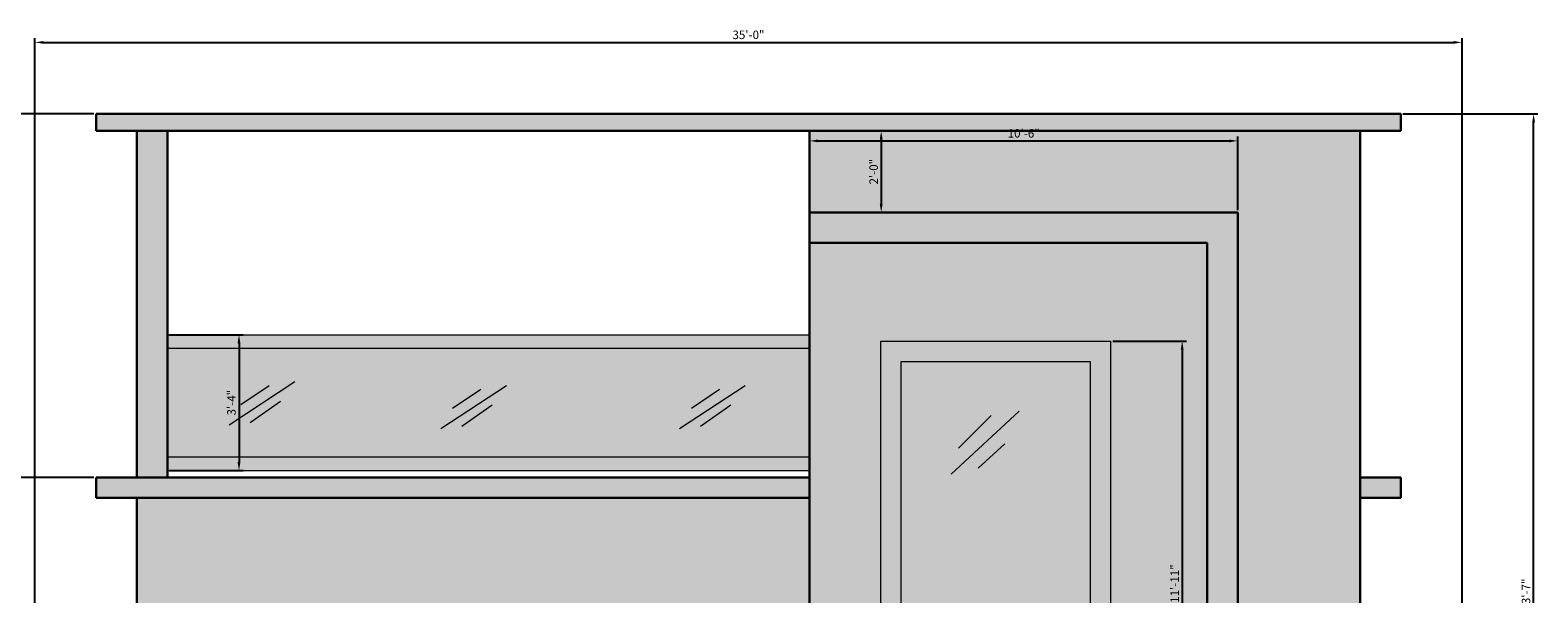
# Model space of a CAD drawing. Units: inches. Extents: x 6038 to 7543, y 3772 to 5131.
# Tile 3 of 14: x 6290 to 6734, y 4063 to 4229. Entities that reach past the tile are written whole.
import ezdxf

# ---------------------------------------------------------------- set-up
doc = ezdxf.new("R2010")
doc.units = ezdxf.units.IN
for name, color, linetype, lineweight in [('A-ANNO-DIMS', 4, 'Continuous', 18), ('A-ELEV', 7, 'Continuous', 30), ('A-ELEV-FRAM-PATT', 7, 'Continuous', 13), ('A-ELEV-GLAZ', 7, 'Continuous', 18)]:
    doc.layers.add(name, color=color, linetype=linetype, lineweight=lineweight)
for name, color, linetype, lineweight, true_color in [('A-ELEV-GLAZ-PATT', 141, 'Continuous', 13, 0xadddf7), ('A-ELEV-METL-PATT', 252, 'Continuous', 13, 0x939598), ('A-ELEV-PANL-PATT', 165, 'Continuous', 13, 0x5e67af), ('A-ELEV-TRIM-PATT', 85, 'Continuous', 13, 0x58ba48), ('A-ELEV-WALL-PATT', 11, 'Continuous', 13, 0xf27172)]:
    doc.layers.add(name, color=color, linetype=linetype, lineweight=lineweight, true_color=true_color)
doc.styles.get("Standard").update_dxf_attribs({"font": 'arial.ttf'})
doc.dimstyles.new('ISO-25', dxfattribs={"dimtxt": 2.5, "dimasz": 2.5, "dimexe": 1.25, "dimexo": 0.625, "dimtad": 1, "dimdec": 0, "dimlunit": 3, "dimtxsty": 'Standard', "dimcen": 2.5, "dimadec": 0, "dimazin": 0, "dimtfac": 1, "dimtdec": 0, "dimtmove": 0, "dimatfit": 3, "dimfxl": 1, "dimarcsym": 0})

# ---------------------------------------------------------------- blocks, each defined once
blk = doc.blocks.new('GLASS-MARK-TALL')
for p, q in [((0, 0), (20.02, 18.51)), ((2.13, 7.66), (11.71, 17.23)), ((7.88, 1.7), (15.76, 8.93))]:
    blk.add_line(p, q)
blk = doc.blocks.new('GLASS-MARK-WIDE')
for p, q in [((0, 0), (19.32, 12.73)), ((3.5, 6.01), (11.76, 11.61)), ((6.16, 0.7), (15.12, 6.99))]:
    blk.add_line(p, q)
blk = doc.blocks.new('*D66')
at = {"layer": 'A-ANNO-DIMS', "color": 0, "lineweight": -2, "transparency": 16777216}
for p, q in [((6291.42, 4008.37), (6291.42, 4227.06)), ((6293.92, 4225.81), (6708.92, 4225.81)), ((6711.42, 4008.37), (6711.42, 4227.06))]:
    blk.add_line(p, q, dxfattribs=at)
at = {"layer": 'A-ANNO-DIMS', "color": 0, "transparency": 16777216}
for points in [[(6293.92, 4226.22), (6293.92, 4225.39), (6291.42, 4225.81)], [(6708.92, 4226.22), (6708.92, 4225.39), (6711.42, 4225.81)]]:
    blk.add_solid(points, dxfattribs=at)
at = {"layer": 'Defpoints', "color": 0, "transparency": 16777216}
for p in [(6711.42, 4225.81), (6291.42, 4007.75), (6711.42, 4007.75)]:
    blk.add_point(p, dxfattribs=at)
at = {"layer": 'A-ANNO-DIMS', "color": 0, "transparency": 16777216, "insert": (6501.42, 4227.71), "char_height": 2.5, "attachment_point": 5}
blk.add_mtext('35\'-0"', dxfattribs=at)
blk = doc.blocks.new('*D67')
at = {"layer": 'A-ANNO-DIMS', "color": 0, "lineweight": -2, "transparency": 16777216}
for p, q in [((6694.04, 4204.75), (6733.73, 4204.75)), ((6732.48, 3924.25), (6732.48, 4202.25)), ((6712.04, 3921.75), (6733.73, 3921.75))]:
    blk.add_line(p, q, dxfattribs=at)
at = {"layer": 'A-ANNO-DIMS', "color": 0, "transparency": 16777216}
for points in [[(6732.06, 4202.25), (6732.89, 4202.25), (6732.48, 4204.75)], [(6732.06, 3924.25), (6732.89, 3924.25), (6732.48, 3921.75)]]:
    blk.add_solid(points, dxfattribs=at)
at = {"layer": 'Defpoints', "color": 0, "transparency": 16777216}
for p in [(6693.42, 4204.75), (6732.48, 4204.75), (6711.42, 3921.75)]:
    blk.add_point(p, dxfattribs=at)
at = {"layer": 'A-ANNO-DIMS', "color": 0, "transparency": 16777216, "insert": (6730.57, 4063.25), "char_height": 2.5, "attachment_point": 5, "rotation": 90}
blk.add_mtext('23\'-7"', dxfattribs=at)
blk = doc.blocks.new('*D75')
at = {"layer": 'A-ANNO-DIMS', "color": 0, "lineweight": -2, "transparency": 16777216}
for p, q in [((6308.79, 4097.75), (6269.11, 4097.75)), ((6270.36, 4010.25), (6270.36, 4095.25)), ((6290.79, 4007.75), (6269.11, 4007.75))]:
    blk.add_line(p, q, dxfattribs=at)
at = {"layer": 'A-ANNO-DIMS', "color": 0, "transparency": 16777216}
for points in [[(6269.94, 4095.25), (6270.77, 4095.25), (6270.36, 4097.75)], [(6269.94, 4010.25), (6270.77, 4010.25), (6270.36, 4007.75)]]:
    blk.add_solid(points, dxfattribs=at)
at = {"layer": 'Defpoints', "color": 0, "transparency": 16777216}
for p in [(6270.36, 4097.75), (6309.42, 4097.75), (6291.42, 4007.75)]:
    blk.add_point(p, dxfattribs=at)
at = {"layer": 'A-ANNO-DIMS', "color": 0, "transparency": 16777216, "insert": (6268.46, 4052.75), "char_height": 2.5, "attachment_point": 5, "rotation": 90}
blk.add_mtext('7\'-6"', dxfattribs=at)
blk = doc.blocks.new('*D76')
at = {"layer": 'A-ANNO-DIMS', "color": 0, "lineweight": -2, "transparency": 16777216}
for p, q in [((6308.79, 4204.75), (6269.11, 4204.75)), ((6270.36, 4100.25), (6270.36, 4202.25)), ((6308.79, 4097.75), (6269.11, 4097.75))]:
    blk.add_line(p, q, dxfattribs=at)
at = {"layer": 'A-ANNO-DIMS', "color": 0, "transparency": 16777216}
for points in [[(6269.94, 4202.25), (6270.77, 4202.25), (6270.36, 4204.75)], [(6269.94, 4100.25), (6270.77, 4100.25), (6270.36, 4097.75)]]:
    blk.add_solid(points, dxfattribs=at)
at = {"layer": 'Defpoints', "color": 0, "transparency": 16777216}
for p in [(6270.36, 4204.75), (6309.42, 4204.75), (6309.42, 4097.75)]:
    blk.add_point(p, dxfattribs=at)
at = {"layer": 'A-ANNO-DIMS', "color": 0, "transparency": 16777216, "insert": (6268.46, 4151.25), "char_height": 2.5, "attachment_point": 5, "rotation": 90}
blk.add_mtext('8\'-11"', dxfattribs=at)
blk = doc.blocks.new('*D77')
at = {"layer": 'A-ANNO-DIMS', "color": 0, "lineweight": -2, "transparency": 16777216}
for p, q in [((6608.62, 4137.88), (6630.3, 4137.88)), ((6629.05, 4135.38), (6629.05, 3997.57)), ((6608.62, 3995.07), (6630.3, 3995.07))]:
    blk.add_line(p, q, dxfattribs=at)
at = {"layer": 'A-ANNO-DIMS', "color": 0, "transparency": 16777216}
for points in [[(6628.64, 4135.38), (6629.47, 4135.38), (6629.05, 4137.88)], [(6628.64, 3997.57), (6629.47, 3997.57), (6629.05, 3995.07)]]:
    blk.add_solid(points, dxfattribs=at)
at = {"layer": 'Defpoints', "color": 0, "transparency": 16777216}
for p in [(6607.99, 4137.88), (6607.99, 3995.07), (6629.05, 3995.07)]:
    blk.add_point(p, dxfattribs=at)
at = {"layer": 'A-ANNO-DIMS', "color": 0, "transparency": 16777216, "insert": (6627.17, 4066.47), "char_height": 2.5, "attachment_point": 5, "rotation": 90}
blk.add_mtext('11\'-11"', dxfattribs=at)
blk = doc.blocks.new('*D79')
at = {"layer": 'A-ANNO-DIMS', "color": 0, "lineweight": -2, "transparency": 16777216}
for p, q in [((6331.04, 4139.75), (6352.73, 4139.75)), ((6351.48, 4137.25), (6351.48, 4102.25)), ((6331.04, 4099.75), (6352.73, 4099.75))]:
    blk.add_line(p, q, dxfattribs=at)
at = {"layer": 'A-ANNO-DIMS', "color": 0, "transparency": 16777216}
for points in [[(6351.06, 4137.25), (6351.89, 4137.25), (6351.48, 4139.75)], [(6351.06, 4102.25), (6351.89, 4102.25), (6351.48, 4099.75)]]:
    blk.add_solid(points, dxfattribs=at)
at = {"layer": 'Defpoints', "color": 0, "transparency": 16777216}
for p in [(6330.42, 4139.75), (6330.42, 4099.75), (6351.48, 4099.75)]:
    blk.add_point(p, dxfattribs=at)
at = {"layer": 'A-ANNO-DIMS', "color": 0, "transparency": 16777216, "insert": (6349.57, 4119.75), "char_height": 2.5, "attachment_point": 5, "rotation": 90}
blk.add_mtext('3\'-4"', dxfattribs=at)
blk = doc.blocks.new('*D80')
at = {"layer": 'A-ANNO-DIMS', "color": 0, "lineweight": -2, "transparency": 16777216}
for p, q in [((6519.42, 4176.37), (6519.42, 4198.06)), ((6645.42, 4176.37), (6645.42, 4198.06)), ((6521.92, 4196.81), (6642.92, 4196.81))]:
    blk.add_line(p, q, dxfattribs=at)
at = {"layer": 'A-ANNO-DIMS', "color": 0, "transparency": 16777216}
for points in [[(6521.92, 4197.22), (6521.92, 4196.39), (6519.42, 4196.81)], [(6642.92, 4197.22), (6642.92, 4196.39), (6645.42, 4196.81)]]:
    blk.add_solid(points, dxfattribs=at)
at = {"layer": 'Defpoints', "color": 0, "transparency": 16777216}
for p in [(6645.42, 4196.81), (6519.42, 4175.75), (6645.42, 4175.75)]:
    blk.add_point(p, dxfattribs=at)
at = {"layer": 'A-ANNO-DIMS', "color": 0, "transparency": 16777216, "insert": (6582.42, 4198.71), "char_height": 2.5, "attachment_point": 5}
blk.add_mtext('10\'-6"', dxfattribs=at)
blk = doc.blocks.new('*D81')
at = {"layer": 'A-ANNO-DIMS', "color": 0, "lineweight": -2, "transparency": 16777216}
for p, q in [((6520.04, 4199.75), (6541.73, 4199.75)), ((6540.48, 4197.25), (6540.48, 4178.25)), ((6520.04, 4175.75), (6541.73, 4175.75))]:
    blk.add_line(p, q, dxfattribs=at)
at = {"layer": 'A-ANNO-DIMS', "color": 0, "transparency": 16777216}
for points in [[(6540.06, 4197.25), (6540.89, 4197.25), (6540.48, 4199.75)], [(6540.06, 4178.25), (6540.89, 4178.25), (6540.48, 4175.75)]]:
    blk.add_solid(points, dxfattribs=at)
at = {"layer": 'Defpoints', "color": 0, "transparency": 16777216}
for p in [(6519.42, 4199.75), (6519.42, 4175.75), (6540.48, 4175.75)]:
    blk.add_point(p, dxfattribs=at)
at = {"layer": 'A-ANNO-DIMS', "color": 0, "transparency": 16777216, "insert": (6538.58, 4187.75), "char_height": 2.5, "attachment_point": 5, "rotation": 90}
blk.add_mtext('2\'-0"', dxfattribs=at)

msp = doc.modelspace()

# ---------------------------------------------------------------- hatches: boundary and pattern name
at = {"layer": 'A-ELEV-FRAM-PATT'}
h = msp.add_hatch(color=256, dxfattribs=at)
h.dxf.hatch_style = 1
h.paths.add_polyline_path([(6607.99, 4137.88), (6540.32, 4137.88), (6540.32, 3995.07), (6607.99, 3995.07)])
h.paths.add_polyline_path([(6546.32, 4131.88), (6601.99, 4131.88), (6601.99, 4001.07), (6546.32, 4001.07), (6546.32, 4007.07)], flags=16)
at = {"layer": 'A-ELEV-GLAZ-PATT'}
h = msp.add_hatch(color=256, dxfattribs=at)
h.dxf.hatch_style = 1
h.paths.add_polyline_path([(6601.99, 4131.88), (6546.32, 4131.88), (6546.32, 4007.07), (6555.42, 4007.07), (6555.42, 4013.07), (6564.42, 4013.07), (6564.42, 4019.07), (6573.42, 4019.07), (6573.42, 4025.07), (6582.42, 4025.07), (6582.42, 4031.07), (6591.42, 4031.07), (6591.42, 4037.07), (6601.99, 4037.07)])
h.paths.add_polyline_path([(6601.99, 4037.07), (6591.42, 4037.07), (6591.42, 4031.07), (6582.42, 4031.07), (6582.42, 4025.07), (6573.42, 4025.07), (6573.42, 4019.07), (6564.42, 4019.07), (6564.42, 4013.07), (6555.42, 4013.07), (6555.42, 4007.07), (6546.32, 4007.07), (6546.32, 4001.07), (6601.99, 4001.07)])
h.paths.add_polyline_path([(6519.42, 4135.75), (6330.42, 4135.75), (6330.42, 4103.75), (6519.42, 4103.75)])
at = {"layer": 'A-ELEV-METL-PATT'}
h = msp.add_hatch(color=256, dxfattribs=at)
h.dxf.hatch_style = 1
h.paths.add_polyline_path([(6519.42, 4139.75), (6330.42, 4139.75), (6330.42, 4135.75), (6519.42, 4135.75)])
h.paths.add_polyline_path([(6519.42, 4103.75), (6330.42, 4103.75), (6330.42, 4099.75), (6519.42, 4099.75)])
h.paths.add_polyline_path([(6469.54, 3993.29), (6462.81, 3993.29), (6462.81, 3951.76), (6469.54, 3951.76)], flags=0)
h.paths.add_polyline_path([(6477.92, 4002.75), (6454.42, 4002.75), (6454.42, 3942.75), (6477.92, 3942.75)])
h.paths.add_polyline_path([(6459.81, 3996.29), (6472.54, 3996.29), (6472.54, 3948.76), (6459.81, 3948.76)], flags=16)
h.paths.add_polyline_path([(6462.81, 3993.29), (6469.54, 3993.29), (6469.54, 3951.76), (6462.81, 3951.76)], flags=0)
h.paths.add_polyline_path([(6503.88, 3993.29), (6497.15, 3993.29), (6497.15, 3951.76), (6503.88, 3951.76)], flags=0)
h.paths.add_polyline_path([(6512.42, 4002.75), (6488.92, 4002.75), (6488.92, 3942.75), (6512.42, 3942.75)])
h.paths.add_polyline_path([(6506.88, 3948.76), (6494.15, 3948.76), (6494.15, 3996.29), (6506.88, 3996.29)], flags=16)
h.paths.add_polyline_path([(6503.88, 3951.76), (6497.15, 3951.76), (6497.15, 3993.29), (6503.88, 3993.29)], flags=0)
at = {"layer": 'A-ELEV-PANL-PATT'}
h = msp.add_hatch(color=256, dxfattribs=at)
h.dxf.hatch_style = 1
h.paths.add_polyline_path([(6438.42, 4003.75), (6297.42, 4003.75), (6297.42, 3926.75), (6438.42, 3926.75)])
h.paths.add_polyline_path([(6705.42, 4003.75), (6681.42, 4003.75), (6681.42, 3926.75), (6705.42, 3926.75)])
h.paths.add_polyline_path([(6711.42, 4003.75), (6705.42, 4003.75), (6705.42, 3926.75), (6711.42, 3926.75)])
h.paths.add_polyline_path([(6297.42, 4003.75), (6291.42, 4003.75), (6291.42, 3926.75), (6297.42, 3926.75)])
h.paths.add_polyline_path([(6330.42, 4199.75), (6321.42, 4199.75), (6321.42, 4097.75), (6330.42, 4097.75)])
h.paths.add_polyline_path([(6636.42, 4166.75), (6519.42, 4166.75), (6519.42, 3935.75), (6636.42, 3935.75)])
h.paths.add_polyline_path([(6607.99, 3995.07), (6540.32, 3995.07), (6540.32, 4137.88), (6607.99, 4137.88)], flags=16)
h.paths.add_polyline_path([(6601.99, 4001.07), (6546.32, 4001.07), (6546.32, 4007.07), (6546.32, 4131.88), (6601.99, 4131.88)], flags=0)
at = {"layer": 'A-ELEV-TRIM-PATT'}
h = msp.add_hatch(color=256, dxfattribs=at)
h.dxf.hatch_style = 1
h.paths.add_polyline_path([(6645.42, 4175.75), (6519.42, 4175.75), (6519.42, 4166.75), (6636.42, 4166.75), (6636.42, 3935.75), (6645.42, 3935.75)])
h.paths.add_polyline_path([(6519.42, 4097.75), (6309.42, 4097.75), (6309.42, 4091.75), (6519.42, 4091.75)])
h.paths.add_polyline_path([(6693.42, 4097.75), (6681.42, 4097.75), (6681.42, 4091.75), (6693.42, 4091.75)])
h.paths.add_polyline_path([(6693.42, 4204.75), (6309.42, 4204.75), (6309.42, 4199.75), (6693.42, 4199.75)])
h.paths.add_polyline_path([(6438.42, 4007.75), (6291.42, 4007.75), (6291.42, 4003.75), (6438.42, 4003.75)])
h.paths.add_polyline_path([(6321.42, 4026.12), (6321.42, 4029.67), (6291.42, 4007.75), (6297.42, 4007.75)])
h.paths.add_polyline_path([(6681.42, 4031.03), (6681.42, 4027.16), (6705.42, 4007.75), (6711.42, 4007.75)])
h.paths.add_polyline_path([(6711.42, 4007.75), (6681.42, 4007.75), (6681.42, 4003.75), (6711.42, 4003.75)])
h.paths.add_polyline_path([(6451.42, 4016.75), (6434.42, 4016.75), (6434.42, 4012.75), (6451.42, 4012.75)])
at = {"layer": 'A-ELEV-WALL-PATT'}
h = msp.add_hatch(color=256, dxfattribs=at)
h.dxf.hatch_style = 1
h.paths.add_polyline_path([(6519.42, 4091.75), (6321.42, 4091.75), (6321.42, 4007.75), (6438.42, 4007.75), (6438.42, 4012.75), (6434.42, 4012.75), (6434.42, 4016.75), (6451.42, 4016.75), (6451.42, 4012.75), (6447.42, 4012.75), (6447.42, 3993.52), (6448.42, 3993.52), (6448.42, 3995.02), (6449.42, 3995.02), (6449.42, 4007.75), (6459.42, 4007.75), (6459.42, 4019.75), (6507.42, 4019.75), (6507.42, 4007.75), (6517.42, 4007.75), (6517.42, 3995.02), (6518.42, 3995.02), (6518.42, 3993.52), (6519.42, 3993.52)])
h.paths.add_polyline_path([(6681.42, 4199.75), (6519.42, 4199.75), (6519.42, 4175.75), (6645.42, 4175.75), (6645.42, 3935.75), (6681.42, 3935.75)])

# ---------------------------------------------------------------- linework, layer by layer
at = {"layer": 'A-ELEV'}
for p, q in [((6309.42, 4204.75), (6693.42, 4204.75)), ((6309.42, 4204.75), (6309.42, 4199.75)), ((6693.42, 4204.75), (6693.42, 4199.75)), ((6309.42, 4199.75), (6693.42, 4199.75)), ((6321.42, 4199.75), (6321.42, 4097.75)), ((6330.42, 4199.75), (6330.42, 4097.75)), ((6519.42, 4199.75), (6519.42, 3935.75)), ((6681.42, 3926.75), (6681.42, 4199.75)), ((6519.42, 4175.75), (6645.42, 4175.75)), ((6645.42, 3935.75), (6645.42, 4175.75)), ((6519.42, 4166.75), (6636.42, 4166.75)), ((6636.42, 3935.75), (6636.42, 4166.75)), ((6309.42, 4097.75), (6519.42, 4097.75)), ((6309.42, 4097.75), (6309.42, 4091.75)), ((6681.42, 4097.75), (6693.42, 4097.75)), ((6693.42, 4097.75), (6693.42, 4091.75)), ((6693.42, 4097.75), (6693.42, 4091.75)), ((6309.42, 4091.75), (6519.42, 4091.75)), ((6321.42, 4091.75), (6321.42, 4007.75)), ((6681.42, 4091.75), (6693.42, 4091.75))]:
    msp.add_line(p, q, dxfattribs=at)
at = {"layer": 'A-ELEV-GLAZ'}
for p, q in [((6330.42, 4139.75), (6519.42, 4139.75)), ((6330.42, 4135.75), (6519.42, 4135.75)), ((6330.42, 4103.75), (6519.42, 4103.75)), ((6330.42, 4099.75), (6519.42, 4099.75))]:
    msp.add_line(p, q, dxfattribs=at)
for points in [[(6540.32, 4137.88), (6607.99, 4137.88), (6607.99, 3995.07), (6540.32, 3995.07)], [(6546.32, 4131.88), (6601.99, 4131.88), (6601.99, 4001.07), (6546.32, 4001.07)]]:
    msp.add_lwpolyline(points, close=True, dxfattribs=at)

# ---------------------------------------------------------------- block references
for name, p in [('GLASS-MARK-WIDE', (6348.56, 4113.23)), ('GLASS-MARK-WIDE', (6410.85, 4112.11)), ('GLASS-MARK-WIDE', (6481.11, 4112.11)), ('GLASS-MARK-TALL', (6561.1, 4098.72))]:
    msp.add_blockref(name, p, dxfattribs=at)

# ---------------------------------------------------------------- dimensions: what is measured, and where the dimension line sits
at = {"layer": 'A-ANNO-DIMS'}
for base, p1, p2, picture, middle in [((6711.42, 4225.81), (6291.42, 4007.75), (6711.42, 4007.75), '*D66', (6501.42, 4227.71)), ((6645.42, 4196.81), (6519.42, 4175.75), (6645.42, 4175.75), '*D80', (6582.42, 4198.71))]:
    dim = msp.add_linear_dim(base=base, p1=p1, p2=p2, dimstyle='ISO-25', override={"dimdec": 1, "dimlfac": 1, "dimrnd": 0, "dimzin": 1, "dimdsep": 46, "dimlunit": 4, "dimfrac": 2}, dxfattribs=at)
    dim.commit()
    dim.dimension.update_dxf_attribs({"geometry": picture, "text_midpoint": middle})
for base, p1, p2, angle, picture, middle in [((6270.36, 4204.75), (6309.42, 4097.75), (6309.42, 4204.75), 90, '*D76', (6268.46, 4151.25)), ((6732.48, 4204.75), (6711.42, 3921.75), (6693.42, 4204.75), 90, '*D67', (6730.57, 4063.25)), ((6540.48, 4175.75), (6519.42, 4199.75), (6519.42, 4175.75), 270, '*D81', (6538.58, 4187.75)), ((6351.48, 4099.75), (6330.42, 4139.75), (6330.42, 4099.75), 270, '*D79', (6349.57, 4119.75)), ((6629.05, 3995.07), (6607.99, 4137.88), (6607.99, 3995.07), 270, '*D77', (6627.17, 4066.47)), ((6270.36, 4097.75), (6291.42, 4007.75), (6309.42, 4097.75), 90, '*D75', (6268.46, 4052.75))]:
    dim = msp.add_linear_dim(base=base, p1=p1, p2=p2, angle=angle, dimstyle='ISO-25', override={"dimdec": 1, "dimlfac": 1, "dimrnd": 0, "dimzin": 1, "dimdsep": 46, "dimlunit": 4, "dimfrac": 2}, dxfattribs=at)
    dim.commit()
    dim.dimension.update_dxf_attribs({"geometry": picture, "text_midpoint": middle})

doc.saveas('drawing.dxf')
